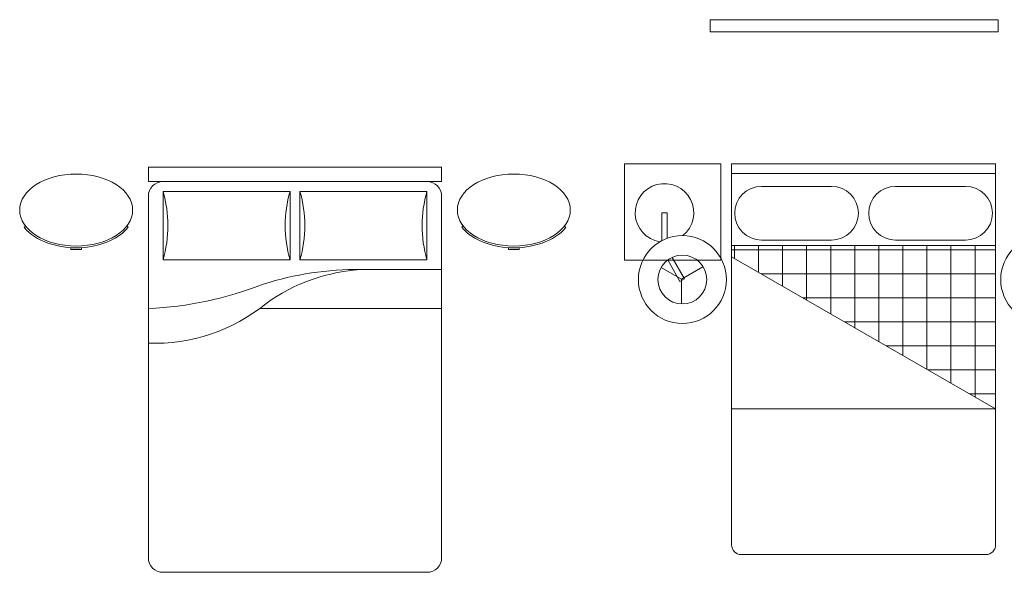
# Model space of a CAD drawing. Units: inches. Extents: x 1994 to 3075, y 3517 to 3950.
# Tile 21 of 58: x 1994.2297 to 1994.4311, y 3553.5867 to 3553.6998. Entities that reach past the tile are written whole.
import ezdxf

# ---------------------------------------------------------------- set-up
doc = ezdxf.new("R2010")
doc.units = ezdxf.units.IN
doc.layers.add('A-FURN-REFR', color=8, linetype='Continuous', lineweight=13)

msp = doc.modelspace()

# ---------------------------------------------------------------- linework, layer by layer
at = {"layer": 'A-FURN-REFR'}
for p, q in [((1994.256040827948, 3553.669659686003), (1994.316040827948, 3553.669659686003)), ((1994.256040827948, 3553.666659686003), (1994.256040827948, 3553.669659686003)), ((1994.316040827948, 3553.666659686003), (1994.316040827948, 3553.669659686003)), ((1994.353465506199, 3553.670297917026), (1994.373150545569, 3553.670297917026)), ((1994.353465506199, 3553.650612877656), (1994.353465506199, 3553.670297917026)), ((1994.373150545569, 3553.670297917026), (1994.373150545569, 3553.650612877656)), ((1994.375345958238, 3553.670297917026), (1994.429345958238, 3553.670297917026)), ((1994.375345958238, 3553.592266420963), (1994.375345958238, 3553.670297917026)), ((1994.429345958238, 3553.670297917026), (1994.429345958238, 3553.592266420963)), ((1994.429345958238, 3553.668297917026), (1994.375345958238, 3553.668297917026)), ((1994.256040827948, 3553.666659686003), (1994.316040827948, 3553.666659686003)), ((1994.395796469914, 3553.665694341239), (1994.381483131362, 3553.665694341239)), ((1994.408895446563, 3553.665694341239), (1994.423208785115, 3553.665694341239)), ((1994.256040827948, 3553.589659686003), (1994.256040827948, 3553.663659686003)), ((1994.259040827948, 3553.664659686003), (1994.259040827948, 3553.650659686003)), ((1994.285040827948, 3553.664659686003), (1994.259040827948, 3553.664659686003)), ((1994.285040827948, 3553.650659686003), (1994.285040827948, 3553.664659686003)), ((1994.313040827948, 3553.664659686003), (1994.287040827948, 3553.664659686003)), ((1994.287040827948, 3553.664659686003), (1994.287040827948, 3553.650659686003)), ((1994.313040827948, 3553.650659686003), (1994.313040827948, 3553.664659686003)), ((1994.316040827948, 3553.663659686003), (1994.316040827948, 3553.589659686003)), ((1994.361092914175, 3553.660302494364), (1994.36106705555, 3553.654561605301)), ((1994.362165220212, 3553.660297664388), (1994.361092914175, 3553.660302494364)), ((1994.36214155526, 3553.655043793864), (1994.362165220212, 3553.660297664388)), ((1994.230949706523, 3553.657544620166), (1994.230651606929, 3553.657311490676)), ((1994.251608569783, 3553.657544620166), (1994.251906669378, 3553.657311490676)), ((1994.320473086112, 3553.657544620166), (1994.320174986518, 3553.657311490676)), ((1994.341131949373, 3553.657544620166), (1994.341430048967, 3553.657311490676)), ((1994.381483131362, 3553.654694341239), (1994.395796469914, 3553.654694341239)), ((1994.423208785115, 3553.654694341239), (1994.408895446563, 3553.654694341239)), ((1994.375345958238, 3553.653599415824), (1994.429345958238, 3553.653599415824)), ((1994.375345958238, 3553.652709904935), (1994.429345958238, 3553.652709904935)), ((1994.375931536125, 3553.653599415824), (1994.375931536125, 3553.650959833475)), ((1994.380852795968, 3553.653599415824), (1994.380852795968, 3553.64811854278)), ((1994.385774055811, 3553.653599415824), (1994.385774055811, 3553.645277252086)), ((1994.390695315653, 3553.653599415824), (1994.390695315653, 3553.64243596139)), ((1994.395616575496, 3553.653599415824), (1994.395616575496, 3553.639594670695)), ((1994.400537835338, 3553.653599415824), (1994.400537835338, 3553.636753380001)), ((1994.405459095181, 3553.653599415824), (1994.405459095181, 3553.633912089306)), ((1994.410380355023, 3553.653599415824), (1994.410380355023, 3553.631070798611)), ((1994.415301614866, 3553.653599415824), (1994.415301614866, 3553.628229507916)), ((1994.420222874708, 3553.653599415824), (1994.420222874708, 3553.625388217221)), ((1994.425144134551, 3553.653599415824), (1994.425144134551, 3553.622546926527)), ((1994.259040827948, 3553.650659686003), (1994.285040827948, 3553.650659686003)), ((1994.287040827948, 3553.650659686003), (1994.313040827948, 3553.650659686003)), ((1994.373150545569, 3553.650612877656), (1994.353465506199, 3553.650612877656)), ((1994.362288204894, 3553.650620749735), (1994.364762799195, 3553.646224954846)), ((1994.36569722633, 3553.646750986684), (1994.36322263203, 3553.651146781573)), ((1994.375345958238, 3553.651297917026), (1994.429345958238, 3553.620121002489)), ((1994.299540827948, 3553.648659686003), (1994.316040827948, 3553.648659686003)), ((1994.365117853428, 3553.646711098967), (1994.360954368829, 3553.649114887921)), ((1994.365117853428, 3553.646711098967), (1994.369447980447, 3553.649211098967)), ((1994.364762799195, 3553.646224954846), (1994.36569722633, 3553.646750986684)), ((1994.365117853428, 3553.646711098967), (1994.365117853428, 3553.641711098967)), ((1994.381424195524, 3553.647788645093), (1994.429345958238, 3553.647788645093)), ((1994.389948067609, 3553.64286738525), (1994.429345958238, 3553.64286738525)), ((1994.279040827948, 3553.640659686003), (1994.316040827948, 3553.640659686003)), ((1994.398471939693, 3553.637946125407), (1994.429345958238, 3553.637946125407)), ((1994.406995811777, 3553.633024865565), (1994.429345958238, 3553.633024865565)), ((1994.415519683862, 3553.628103605723), (1994.429345958238, 3553.628103605723)), ((1994.424043555947, 3553.62318234588), (1994.429345958238, 3553.62318234588)), ((1994.429345958238, 3553.620121002489), (1994.375345958238, 3553.620121002489)), ((1994.427377454301, 3553.590297917025), (1994.377314462175, 3553.590297917025)), ((1994.313040827948, 3553.586659686003), (1994.259040827948, 3553.586659686003))]:
    msp.add_line(p, q, dxfattribs=at)
msp.add_lwpolyline([(1994.370993535893, 3553.699832302582), (1994.429881082485, 3553.699832302582), (1994.429881082485, 3553.697353107878), (1994.370993535893, 3553.697353107878)], close=True, dxfattribs=at)
for points in [[(1994.242390765916, 3553.653130612717), (1994.242390765916, 3553.652792143244), (1994.240164088765, 3553.652792143244), (1994.240164088765, 3553.65314206756)], [(1994.32969088998, 3553.653130612717), (1994.32969088998, 3553.652792143244), (1994.331917567131, 3553.652792143244), (1994.331917567131, 3553.65314206756)]]:
    msp.add_lwpolyline(points, dxfattribs=at)
for centre, radius in [((1994.36528119759, 3553.646609183854), 0.009), ((1994.439410718887, 3553.646609183854), 0.009), ((1994.36528119759, 3553.646609183854), 0.005)]:
    msp.add_circle(centre, radius, dxfattribs=at)
for centre, radius, start, end in [((1994.259040827948, 3553.663659686003), 0.003, 90, 180), ((1994.313040827948, 3553.663659686003), 0.003, 0, 90), ((1994.361620943552, 3553.660269437891), 0.006, 309.0280450997005, 260.9719549002175), ((1994.381483131362, 3553.660194341239), 0.0055000000000002, 90, 270), ((1994.395796469914, 3553.660194341239), 0.005499999999998, 270, 90), ((1994.408895446563, 3553.660194341239), 0.005499999999998, 90, 270), ((1994.423208785115, 3553.660194341239), 0.0055000000000002, 270, 90), ((1994.235040827948, 3553.657659686003), 0.025, 343.7397950002315, 16.26020499976852), ((1994.309040827948, 3553.657659686003), 0.025, 163.7397950002315, 196.2602049997685), ((1994.263040827948, 3553.657659686003), 0.025, 343.7397950002315, 16.26020499976852), ((1994.337040827948, 3553.657659686003), 0.025, 163.7397950002315, 196.2602049997685), ((1994.298728327948, 3553.585909686003), 0.06275526, 89.2581639999226, 107.8033669998943), ((1994.301669859948, 3553.611933880004), 0.036761918, 92.5397819999739, 126.0403109999258), ((1994.252682131948, 3553.714170556003), 0.073587559, 272.616011999866, 291.4069440001082), ((1994.257540827948, 3553.668909686003), 0.035338541, 267.5672600000702, 309.5460809998612), ((1994.377314462175, 3553.592266420963), 0.0019685039370083, 180, 270), ((1994.427377454301, 3553.592266420963), 0.0019685039370083, 270, 0), ((1994.259040827948, 3553.589659686003), 0.003, 180, 270), ((1994.313040827948, 3553.589659686003), 0.003, 270, 0)]:
    msp.add_arc(centre, radius, start, end, dxfattribs=at)
msp.add_ellipse((1994.241279138153, 3553.660848915975), major_axis=(-0.0115547702868297, 0), ratio=0.6380952262439872, dxfattribs=at)
at = {"layer": 'A-FURN-REFR', "extrusion": (0, 0, -1)}
msp.add_ellipse((1994.330802517742, 3553.660848915975), major_axis=(0.0115547702868297, 0), ratio=0.6380952262439874, dxfattribs=at)
at = {"layer": 'A-FURN-REFR'}
for points in [[(1994.230651606929, 3553.657311490676), (1994.230803137806, 3553.657117730149), (1994.230966956133, 3553.656928661515), (1994.233590098011, 3553.654186679484), (1994.23839625113, 3553.652762941425), (1994.246688343924, 3553.653508483705), (1994.250118125487, 3553.655098912826), (1994.251898497353, 3553.657317881627)], [(1994.341430048967, 3553.657311490676), (1994.34127851809, 3553.657117730149), (1994.341114699763, 3553.656928661515), (1994.338491557885, 3553.654186679484), (1994.333685404765, 3553.652762941425), (1994.325393311972, 3553.653508483705), (1994.321963530409, 3553.655098912826), (1994.320183158543, 3553.657317881627)]]:
    msp.add_open_spline(points, degree=3, knots=[0.4646241215487272, 0.4646241215487272, 0.4646241215487272, 0.4646241215487272, 0.5480603081879517, 0.5480603081879517, 1.710778559552908, 1.710778559552908, 2.676846635121382, 2.676846635121382, 2.676846635121382, 2.676846635121382], dxfattribs=at)

doc.saveas('drawing.dxf')
